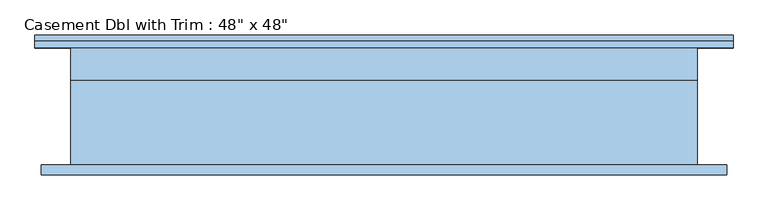
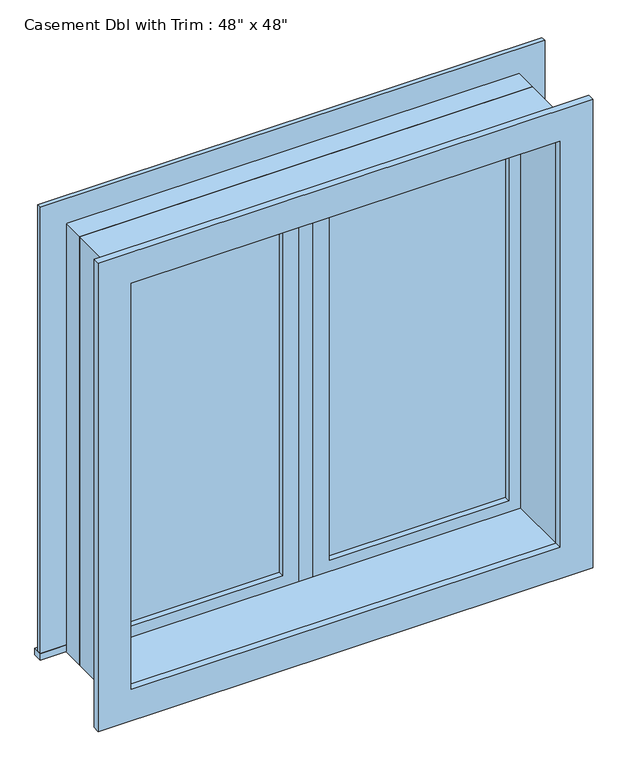
"""IFC4 building model written with IfcOpenShell, lengths in millimetres: window geometry."""

from ifc_helpers import new_model, si_unit, frame, origin, place, context, project, spatial, polyline, outline, extrude, source, transform, mapped, element, save


def window_534dcd48(model_context):
    return source(origin(), model_context, "Body", "SweptSolid", [
        extrude(outline(polyline([(63.5, 98.425), (546.1, 98.425), (546.1, 85.725), (63.5, 85.725), (63.5, 98.425)])), frame((0.0, 0.0, 977.9), z_axis=(0.0, 0.0, 1.0), x_axis=(1.0, 0.0, 0.0)), (0.0, 0.0, 1.0), 1092.2),
        extrude(outline(polyline([(2114.55, 19.05), (933.45, 19.05), (933.45, 590.55), (2114.55, 590.55), (2114.55, 19.05)]), holes=[polyline([(2070.1, 63.5), (2070.1, 546.1), (977.9, 546.1), (977.9, 63.5), (2070.1, 63.5)])]), frame((0.0, 69.85, 0.0), z_axis=(0.0, 1.0, 0.0), x_axis=(0.0, 0.0, 1.0)), (0.0, 0.0, 1.0), 44.45),
        extrude(outline(polyline([(19.05, 69.85), (-19.05, 69.85), (-19.05, 133.35), (19.05, 133.35), (19.05, 69.85)])), frame((0.0, 0.0, 933.45), z_axis=(0.0, 0.0, 1.0), x_axis=(1.0, 0.0, 0.0)), (0.0, 0.0, 1.0), 1181.1),
        extrude(outline(polyline([(-679.45, 158.75), (679.45, 158.75), (679.45, 133.35), (-679.45, 133.35), (-679.45, 158.75)])), frame((0.0, 0.0, 914.4), z_axis=(0.0, 0.0, 1.0), x_axis=(1.0, 0.0, 0.0)), (0.0, 0.0, 1.0), 19.05),
        extrude(outline(polyline([(2114.55, -590.55), (2114.55, 590.55), (933.45, 590.55), (933.45, 679.45), (2203.45, 679.45), (2203.45, -679.45), (933.45, -679.45), (933.45, -590.55), (2114.55, -590.55)])), frame((0.0, 133.35, 0.0), z_axis=(0.0, 1.0, 0.0), x_axis=(0.0, 0.0, 1.0)), (0.0, 0.0, 1.0), 12.7),
        extrude(outline(polyline([(2190.75, 666.75), (2190.75, -666.75), (857.25, -666.75), (857.25, 666.75), (2190.75, 666.75)]), holes=[polyline([(2101.85, 577.85), (946.15, 577.85), (946.15, -577.85), (2101.85, -577.85), (2101.85, 577.85)])]), frame((0.0, -114.3, 0.0), z_axis=(0.0, 1.0, 0.0), x_axis=(0.0, 0.0, 1.0)), (0.0, 0.0, 1.0), 19.05),
        extrude(outline(polyline([(-63.5, 85.725), (-546.1, 85.725), (-546.1, 98.425), (-63.5, 98.425), (-63.5, 85.725)])), frame((0.0, 0.0, 977.9), z_axis=(0.0, 0.0, 1.0), x_axis=(1.0, 0.0, 0.0)), (0.0, 0.0, 1.0), 1092.2),
        extrude(outline(polyline([(2114.55, -590.55), (933.45, -590.55), (933.45, -19.05), (2114.55, -19.05), (2114.55, -590.55)]), holes=[polyline([(2070.1, -546.1), (2070.1, -63.5), (977.9, -63.5), (977.9, -546.1), (2070.1, -546.1)])]), frame((0.0, 69.85, 0.0), z_axis=(0.0, 1.0, 0.0), x_axis=(0.0, 0.0, 1.0)), (0.0, 0.0, 1.0), 44.45),
        extrude(outline(polyline([(2133.6, -609.6), (914.4, -609.6), (914.4, 609.6), (2133.6, 609.6), (2133.6, -609.6)]), holes=[polyline([(2101.85, -577.85), (2101.85, 577.85), (946.15, 577.85), (946.15, -577.85), (2101.85, -577.85)])]), frame((0.0, -95.25, 0.0), z_axis=(0.0, 1.0, 0.0), x_axis=(0.0, 0.0, 1.0)), (0.0, 0.0, 1.0), 165.1),
        extrude(outline(polyline([(2133.6, 609.6), (2133.6, -609.6), (914.4, -609.6), (914.4, 609.6), (2133.6, 609.6)]), holes=[polyline([(2114.55, 590.55), (933.45, 590.55), (933.45, -590.55), (2114.55, -590.55), (2114.55, 590.55)])]), frame((0.0, 69.85, 0.0), z_axis=(0.0, 1.0, 0.0), x_axis=(0.0, 0.0, 1.0)), (0.0, 0.0, 1.0), 63.5),
    ])


if __name__ == "__main__":
    model = new_model("IFC4")
    model_context = context("Model", 3, world=origin())
    ifc_project = project(units=[si_unit("LENGTHUNIT", "METRE", prefix="MILLI")], contexts=[model_context])
    site = spatial("IfcSite", under=ifc_project)
    building = spatial("IfcBuilding", under=site)
    placement = place(None, origin())
    window_shape = window_534dcd48(model_context)
    element("IfcWindow", 1, ObjectType="Casement Dbl with Trim : 48\" x 48\"", at=placement, inside=building, context=model_context, shape_type="MappedRepresentation", body=[
        mapped(window_shape, transform((0.0, 0.0, 0.0), x_axis=(1.0, 0.0, 0.0), y_axis=(0.0, 1.0, 0.0), z_axis=(0.0, 0.0, 1.0))),
    ])
    save(model, "model.ifc")

# Revit data of these elements
# Type "Casement Dbl with Trim : 48\" x 48\""
#   Type Mark = "10"
#   Construction Type Id = "GSP4R"
#   Assembly Code = "B2020100"
#   Analytic Construction = "1/8 in Pilkington single glazing"
#   Visual Light Transmittance = 0.9
#   Solar Heat Gain Coefficient = 0.78
#   Heat Transfer Coefficient (U) = 0.6496 BTU/(h·ft²·°F)
#   Height = 4' - 0"
#   Default Sill Height = 3' - 0"
#   Trim Projection - Ext. = 0' - 0 1/2"
#   Trim Projection - Int. = 0' - 0 3/4"
#   Trim Width - Exterior = 0' - 3 1/2"
#   Trim Width - Interior = 0' - 3 1/2"
#   Width = 4' - 0"
#   Window Inset = 0' - 0 3/4"
#   Define Thermal Properties by = 1
#   Glass Pane Material = Glass
#   Sash Material = Sash
#   Trim Exterior Material = Trim
#   Trim Interior Material = Trim
#   Wall Closure = (empty or 0)
# Element 1 (IfcWindow, "Casement Dbl with Trim : 48\" x 48\"")
#   Materials on its faces: "Sash", "Trim", "Glass"
# Materials
#   "Glass": class "Glass", colour RGB 0 128 192, transparency 0.75, Description = "Soda Lime Glass", Cost = 0
#   "Sash": class "Wood", colour RGB 224 178 126, transparency 0
#   "Trim": class "Wood", colour RGB 224 178 126, transparency 0
